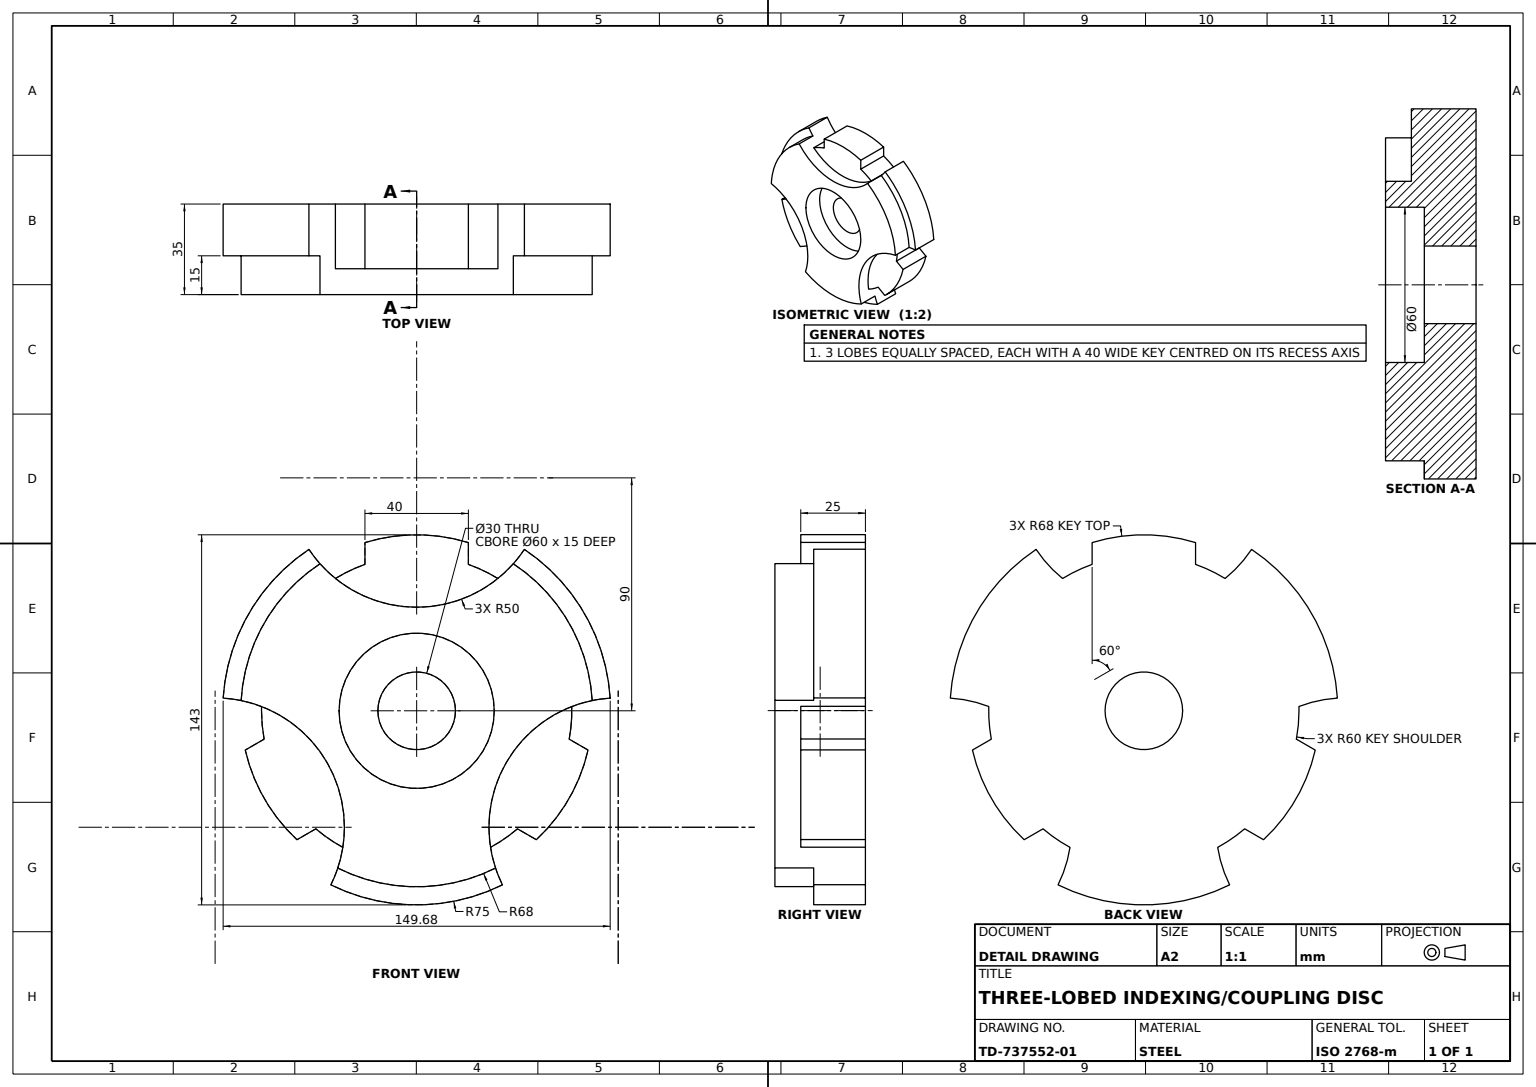
SolidWorks part; units mm, degrees
material "Plain Carbon Steel"
ref_plane "Front Plane" through (0, 0, 0) normal (0, 0, 1) x (1, 0, 0)
ref_plane "Top Plane" through (0, 0, 0) normal (0, 1, 0) x (1, 0, 0)
ref_plane "Right Plane" through (0, 0, 0) normal (1, 0, 0) x (0, 0, -1)
sketch "Base Disc Sketch" plane through (0, 0, 0) normal (0, 0, 1) x (1, 0, 0)
  circle A0 centre (0, 0) radius 90 construction
  circle A1 centre (0, 0) radius 75
  dimension "D1" = 90
  dimension "D2" = 75
extrude "Base Disc" add sketch "Base Disc Sketch" along normal blind 20
sketch "Hub Boss Sketch" plane through (0, 0, 20) normal (0, 0, 1) x (1, 0, 0)
  circle A0 centre (0, 0) radius 68
  dimension "D1" = 68
extrude "Hub Boss" add sketch "Hub Boss Sketch" along normal blind 15
sketch "Lobe Recess Sketch" plane through (0, 0, 35) normal (0, 0, 1) x (1, 0, 0)
  line L0 (0, 0) -> (0, 68)
  line L1 (0, 0) -> (0, -68)
  line L2 (-68, 0) -> (68, 0)
  line L3 (0, 0) -> (58.8897, -34)
  line L4 (0, 0) -> (-58.8897, -34)
  line L5 (0, 68) -> (0, 90)
  line L6 (-58.8897, -34) -> (-77.9423, -45)
  line L7 (58.8897, -34) -> (77.9423, -45)
  circle A0 centre (0, 0) radius 68 construction
  circle A1 centre (0, 0) radius 68 construction
  circle A2 centre (0, 0) radius 68
  circle A3 centre (0, 0) radius 90
  circle A4 centre (-77.9423, -45) radius 50
  circle A5 centre (77.9423, -45) radius 50
  circle A6 centre (0, 90) radius 50
  circle M4 centre (0, 0) radius 68
  dimension "D1" = 60
  dimension "D3" = 68
  dimension "D4" = 90
  dimension "D5" = 100
  dimension "D6" = 100
  dimension "D7" = 100
  dimension "D2" = 60
extrude "Lobe Recess Cut" cut sketch "Lobe Recess Sketch" against normal blind 35 contours A3 A6 L5 M4 | A6 A3 L5 M4 | L0 A6 M4 | A6 L0 M4 | A3 A5 L7 M4 | A2 A5 A3 L7 | L2 A5 L3 M4 | L3 A5 A2 | A5 L2 M4 | A2 A4 A3 L6 M4 | L4 A4 L2 M4 | A4 L4 M4 | A3 A4 L6 M4 | L2 A4 A2
sketch "Coupling Lobes Sketch" plane through (0, 0, 0) normal (0, 0, -1) x (-1, 0, 0)
  line L0 (0, 0) -> (0, 68)
  line L1 (58.9898, -10.9638) -> (66.285, -15.1756)
  line L2 (20, 64.9923) -> (20, 56.5685)
  line L3 (-38.9898, -45.6048) -> (-46.285, -49.8167)
  line L4 (-20, 56.5685) -> (-20, 64.9923)
  line L5 (46.285, -49.8167) -> (38.9898, -45.6048)
  line L6 (-66.285, -15.1756) -> (-58.9898, -10.9638)
  arc A0 (20, 64.9923) -> (-20, 64.9923) centre (0, 0) ccw
  arc A1 (-20, 56.5685) -> (-31.427, 51.1111) centre (0, 0) ccw
  arc A2 (-38.9898, -45.6048) -> (-28.55, -52.7721) centre (0, 0) ccw
  arc A3 (58.9898, -10.9638) -> (59.977, 1.661) centre (0, 0) ccw
  arc A4 (-66.285, -15.1756) -> (-46.285, -49.8167) centre (0, 0) ccw
  arc A5 (46.285, -49.8167) -> (66.285, -15.1756) centre (0, 0) ccw
  arc A6 (-31.427, 51.1111) -> (31.427, 51.1111) centre (0, 90) ccw
  arc A7 (-59.977, 1.661) -> (-28.55, -52.7721) centre (-77.9423, -45) cw
  arc A8 (28.55, -52.7721) -> (59.977, 1.661) centre (77.9423, -45) cw
  arc A9 (31.427, 51.1111) -> (20, 56.5685) centre (0, 0) ccw
  arc A10 (-59.977, 1.661) -> (-58.9898, -10.9638) centre (0, 0) ccw
  arc A11 (28.55, -52.7721) -> (38.9898, -45.6048) centre (0, 0) ccw
  arc M9 (41.6664, 62.3611) -> (-41.6664, 62.3611) centre (0, 90) cw
  arc M11 (-74.8395, 4.9036) -> (-33.1731, -67.2647) centre (-77.9423, -45) cw
  arc M13 (33.1731, -67.2647) -> (74.8395, 4.9036) centre (77.9423, -45) cw
  dimension "D1" = 68
  dimension "D2" = 60
  dimension "D7" = 49.4501
  dimension "D8" = 50
  dimension "D14" = 50
  dimension "D15" = 50
  dimension "D3" = 3
  dimension "D4" = 3
  dimension "D5" = 40
  dimension "D6" = 20
  dimension "D9" = 103.8832
  dimension "D10" = 59.977
  dimension "D11" = 91.404
  dimension "D12" = 103.8832
  dimension "D13" = 119.954
extrude "Coupling Lobes" add sketch "Coupling Lobes Sketch" against normal blind 25 contours L4 A1 L0 A0 M9 | A9 L2 A0 L0 M9 | A10 L6 A4 L3 A2 M11 | A11 L5 A5 L1 A3 M13
sketch "Counterbore Sketch" plane through (0, 0, 35) normal (0, 0, 1) x (1, 0, 0)
  circle A0 centre (0, 0) radius 30
  dimension "D1" = 30
extrude "Counterbore" cut sketch "Counterbore Sketch" against normal blind 15
sketch "Through Bore Sketch" plane through (0, 0, 20) normal (0, 0, 1) x (1, 0, 0)
  circle A0 centre (0, 0) radius 15
  dimension "D1" = 15
extrude "Through Bore" cut sketch "Through Bore Sketch" against normal blind 20
